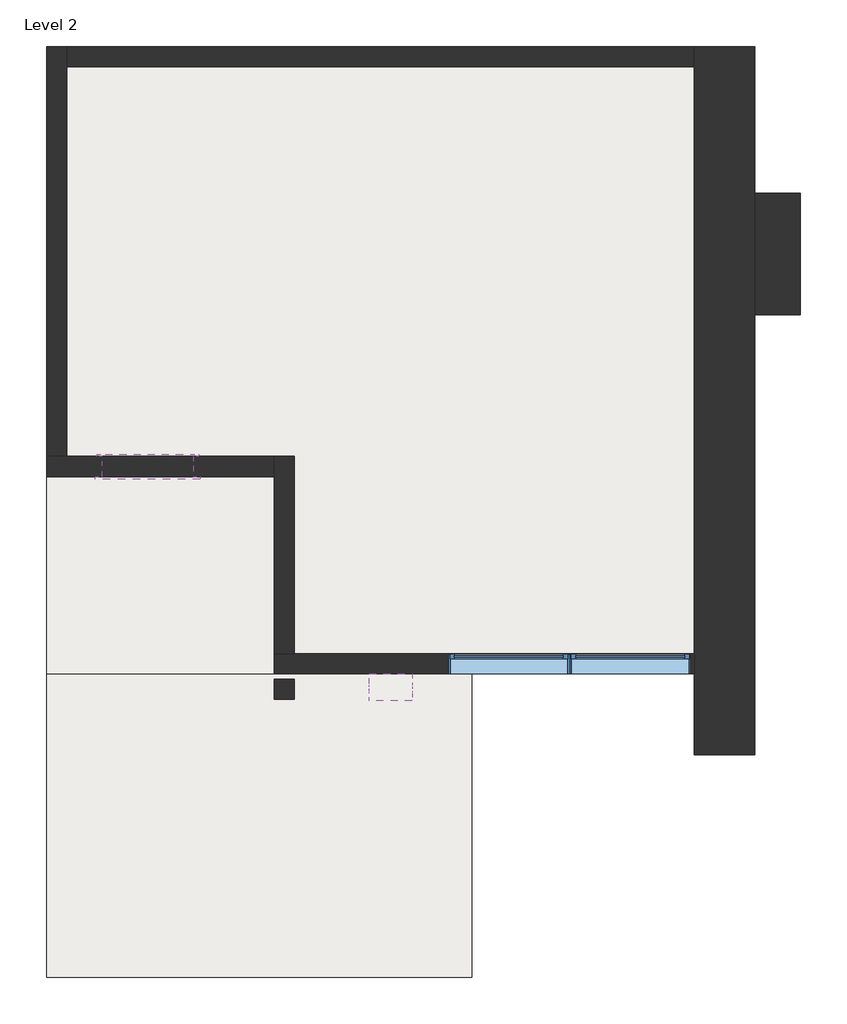
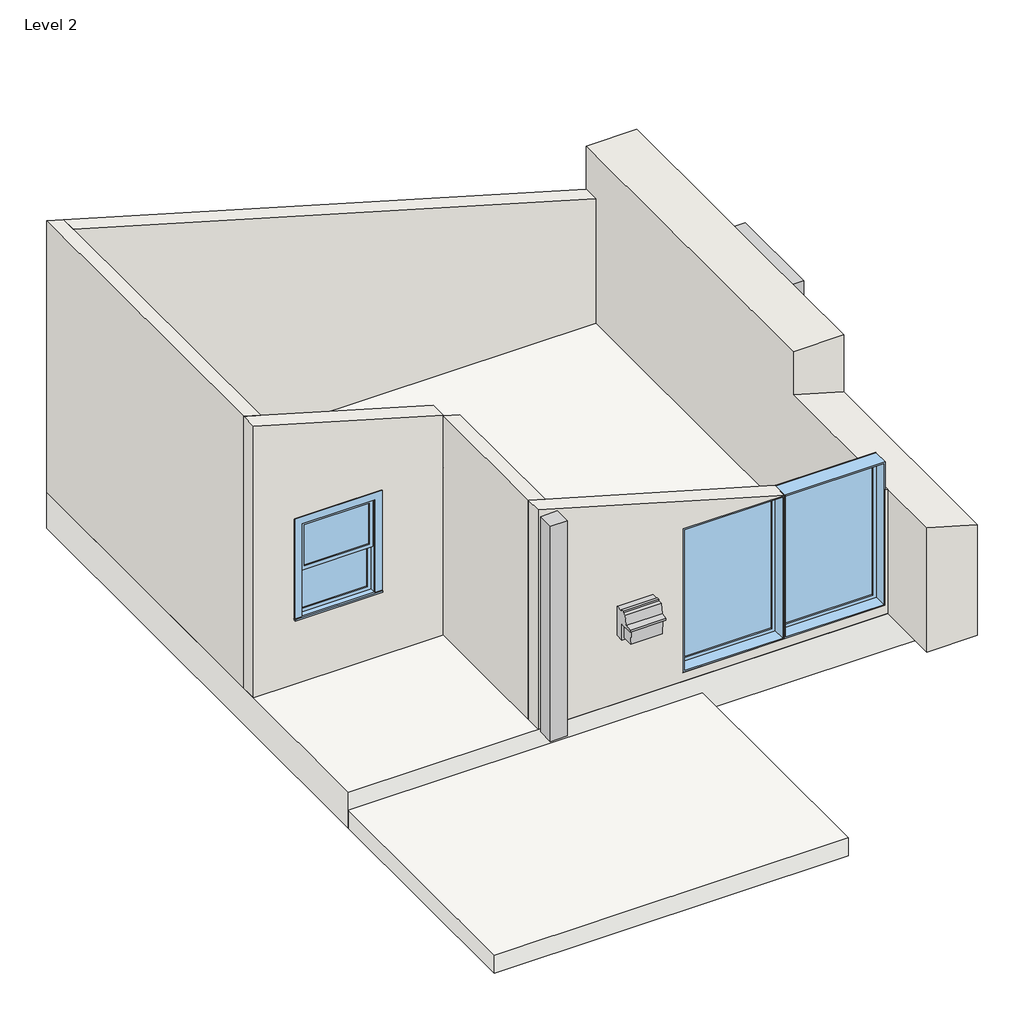
# One storey: 6 walls, 3 windows, 2 columns, 2 roofs, 1 light fixture.
"""IFC4 building model written with IfcOpenShell, lengths in millimetres."""

from ifc_helpers import new_model, si_unit, frame, origin, place, context, project, spatial, polyline, outline, extrude, faceted_brep, transform, mapped, element, save
from components import wall_pack_light_exterior_120v_50d39a1a, window_31198920, window_b4876e44

model = new_model("IFC4")

# Units and contexts
model_context = context("Model", 3, world=origin())
ifc_project = project(units=[si_unit("LENGTHUNIT", "METRE", prefix="MILLI")], contexts=[model_context])

# Site, building, storey
site = spatial("IfcSite", under=ifc_project)
building = spatial("IfcBuilding", under=site)
storey = spatial("IfcBuildingStorey", under=building, Name="Level 2", Elevation=3048.0)

# Columns
placement = place(None, origin())
element("IfcColumn", 1, ObjectType="Rectangular Column : 18\" x 18\"", at=placement, inside=storey, context=model_context, shape_type="SweptSolid", body=[
    extrude(outline(polyline([(-18066.8304544, -4040.8287936), (-18066.8304544, -4244.0287936), (-18270.0304544, -4244.0287936), (-18270.0304544, -4040.8287936), (-18066.8304544, -4040.8287936)])), frame((0.0, 0.0, 3505.2), z_axis=(0.0, 0.0, 1.0), x_axis=(1.0, 0.0, 0.0)), (0.0, 0.0, 1.0), 2743.2),
])
element("IfcColumn", 2, ObjectType="Rectangular Column : 24\" x 24\"", at=placement, inside=storey, context=model_context, shape_type="SweptSolid", body=[
    extrude(outline(polyline([(3048.0, -13901.2613196), (3048.0, -12986.8613196), (5181.6, -12986.8613196), (5181.6, -13444.0613196), (3505.2, -13444.0613196), (3505.2, -13901.2613196), (3048.0, -13901.2613196)])), frame((0.0, -381.4582127, 0.0), z_axis=(0.0, 1.0, 0.0), x_axis=(0.0, 0.0, 1.0)), (0.0, 0.0, 1.0), 1219.2),
])

# Light fixture
wall_pack_light_exterior_120v_shape = wall_pack_light_exterior_120v_50d39a1a(model_context)
element("IfcLightFixture", 3, ObjectType="Wall Pack Light - Exterior : 120V", at=placement, inside=storey, context=model_context, shape_type="MappedRepresentation", body=[
    mapped(wall_pack_light_exterior_120v_shape, transform((-16979.8972631, -3886.6582127, 1996.0613502), x_axis=(-1.0, 0.0, 0.0), y_axis=(0.0, -1.0, 0.0), z_axis=(0.0, 0.0, 1.0))),
])

# Roofs
element("IfcRoof", 4, ObjectType="Generic - 18\" 2", at=placement, inside=storey, context=model_context, shape_type="SweptSolid", body=[
    extrude(outline(polyline([(-20556.0613196, 2310.9417873), (-13444.0613196, 2310.9417873), (-13444.0613196, -3988.2582127), (-20556.0613196, -3988.2582127), (-20556.0613196, 2310.9417873)])), frame((0.0, 0.0, 3048.0), z_axis=(0.0, 0.0, 1.0), x_axis=(1.0, 0.0, 0.0)), (0.0, 0.0, 1.0), 457.2),
])
element("IfcRoof", 5, ObjectType="Generic - 9\"", at=placement, inside=storey, context=model_context, shape_type="SweptSolid", body=[
    extrude(outline(polyline([(-20556.0613196, -3988.2582127), (-16288.8613196, -3988.2582127), (-16288.8613196, -7036.2582127), (-20556.0613196, -7036.2582127), (-20556.0613196, -3988.2582127)])), frame((0.0, 0.0, 3048.0), z_axis=(0.0, 0.0, 1.0), x_axis=(1.0, 0.0, 0.0)), (0.0, 0.0, 1.0), 228.6),
])

# Walls
element("IfcWall", 6, ObjectType="Generic - 8\"", at=placement, inside=storey, context=model_context, shape_type="Brep", body=[
    faceted_brep([(-14053.6613196, -3785.0582127, 3505.2), (-18066.8613196, -3785.0582127, 3505.2), (-18270.0613196, -3785.0582127, 3505.2), (-18270.0613196, -3785.0582127, 6301.6044651), (-18066.8613196, -3785.0582127, 6243.2365005), (-15293.901566, -3785.0582127, 5446.7206706), (-16523.9413429, -3785.0582127, 5446.7206706), (-16523.9413429, -3785.0582127, 3617.9206706), (-14085.5413429, -3785.0582127, 3617.9206706), (-14085.5413429, -3785.0582127, 5099.6265433), (-14053.6613196, -3785.0582127, 5090.4692004), (-18270.0613196, -3988.2582127, 3505.2), (-14053.6613196, -3988.2582127, 3505.2), (-14053.6613196, -3988.2582127, 5090.4692004), (-14085.5413429, -3988.2582127, 5099.6265433), (-14085.5413429, -3988.2582127, 3617.9206706), (-16523.9413429, -3988.2582127, 3617.9206706), (-16523.9413429, -3988.2582127, 5446.7206706), (-15293.901566, -3988.2582127, 5446.7206706), (-18270.0613196, -3988.2582127, 6301.6044651)], [[[0, 1, 2, 3, 4, 5, 6, 7, 8, 9, 10]], [[11, 12, 13, 14, 15, 16, 17, 18, 19]], [[2, 1, 0, 12, 11]], [[3, 2, 11, 19]], [[0, 10, 13, 12]], [[8, 15, 14, 9]], [[16, 7, 6, 17]], [[7, 16, 15, 8]], [[17, 6, 5, 18]], [[3, 19, 18, 5, 4]], [[13, 10, 9, 14]]]),
])
element("IfcWall", 7, ObjectType="Generic - 8\"", at=placement, inside=storey, context=model_context, shape_type="Brep", body=[
    faceted_brep([(-18066.8613196, -3785.0582127, 3505.2), (-18066.8613196, -1803.8582127, 3505.2), (-18066.8613196, -1803.8582127, 5638.8), (-18066.8613196, -2007.0582127, 5638.8), (-18066.8613196, -2007.0582127, 6243.2365005), (-18066.8613196, -3785.0582127, 6243.2365005), (-18270.0613196, -3785.0582127, 3505.2), (-18270.0613196, -3785.0582127, 6301.6044651), (-18270.0613196, -2007.0582127, 6301.6044651), (-18270.0613196, -2007.0582127, 5638.8), (-18270.0613196, -1803.8582127, 5638.8), (-18270.0613196, -1803.8582127, 3505.2), (-18270.0613196, -2007.0582127, 3505.2)], [[[0, 1, 2, 3, 4, 5]], [[6, 7, 8, 9, 10, 11, 12]], [[1, 0, 6, 12, 11]], [[0, 5, 7, 6]], [[2, 1, 11, 10]], [[3, 2, 10, 9]], [[3, 9, 8, 4]], [[5, 4, 8, 7]]]),
])
element("IfcWall", 8, ObjectType="Generic - 8\"", at=placement, inside=storey, context=model_context, shape_type="Brep", body=[
    faceted_brep([(-18270.0613196, -1803.8582127, 3505.2), (-20352.8613196, -1803.8582127, 3505.2), (-20556.0613196, -1803.8582127, 3505.2), (-20556.0613196, -1803.8582127, 6966.6625001), (-20352.8613196, -1803.8582127, 6908.0886191), (-18270.0613196, -1803.8582127, 6307.7063391), (-18270.0613196, -1803.8582127, 5638.8), (-19997.2613196, -1803.8582127, 5544.8047365), (-19997.2613196, -1803.8582127, 4325.6047365), (-19082.8613196, -1803.8582127, 4325.6047365), (-19082.8613196, -1803.8582127, 5544.8047365), (-18270.0613196, -2007.0582127, 3505.2), (-18270.0613196, -2007.0582127, 6307.7063391), (-20556.0613196, -2007.0582127, 6966.6625001), (-20556.0613196, -2007.0582127, 3505.2), (-19997.2613196, -2007.0582127, 5544.8047365), (-19082.8613196, -2007.0582127, 5544.8047365), (-19082.8613196, -2007.0582127, 4325.6047365), (-19997.2613196, -2007.0582127, 4325.6047365)], [[[0, 1, 2, 3, 4, 5, 6], [7, 8, 9, 10]], [[11, 12, 13, 14], [15, 16, 17, 18]], [[2, 1, 0, 11, 14]], [[0, 6, 5, 12, 11]], [[3, 2, 14, 13]], [[5, 4, 3, 13, 12]], [[8, 7, 15, 18]], [[9, 8, 18, 17]], [[10, 9, 17, 16]], [[7, 10, 16, 15]]]),
])
element("IfcWall", 9, ObjectType="Generic - 8\"", at=placement, inside=storey, context=model_context, shape_type="Brep", body=[
    faceted_brep([(-20352.8613196, -1803.8582127, 3505.2), (-20352.8613196, 2107.7417873, 3505.2), (-20352.8613196, 2310.9417873, 3505.2), (-20352.8613196, 2310.9417873, 6908.0886191), (-20352.8613196, 2107.7417873, 6908.0886191), (-20352.8613196, -1803.8582127, 6908.0886191), (-20556.0613196, -1803.8582127, 3505.2), (-20556.0613196, -1803.8582127, 6966.6625001), (-20556.0613196, 2310.9417873, 6966.6625001), (-20556.0613196, 2310.9417873, 3505.2)], [[[0, 1, 2, 3, 4, 5]], [[6, 7, 8, 9]], [[2, 1, 0, 6, 9]], [[0, 5, 7, 6]], [[3, 2, 9, 8]], [[5, 4, 3, 8, 7]]]),
])
element("IfcWall", 10, ObjectType="Generic - 8\"", at=placement, inside=storey, context=model_context, shape_type="SweptSolid", body=[
    extrude(outline(polyline([(3505.2, -20352.8613196), (3505.2, -14053.6613196), (5092.2983086, -14053.6613196), (6908.0886191, -20352.8613196), (3505.2, -20352.8613196)])), frame((0.0, 2107.7417873, 0.0), z_axis=(0.0, 1.0, 0.0), x_axis=(0.0, 0.0, 1.0)), (0.0, 0.0, 1.0), 203.2),
])
element("IfcWall", 11, ObjectType="Generic - 8\" 2", at=placement, inside=storey, context=model_context, shape_type="Brep", body=[
    faceted_brep([(-14053.6613196, 2310.9417873, 3505.2), (-14053.6613196, 2107.7417873, 3505.2), (-14053.6613196, -3785.0582127, 3505.2), (-14053.6613196, -3988.2582127, 3505.2), (-14053.6613196, -4801.0582127, 3505.2), (-14053.6613196, -4801.0582127, 5090.4692004), (-14053.6613196, -3988.2582127, 5090.4692004), (-14053.6613196, -3785.0582127, 5090.4692004), (-14053.6613196, -2007.0582127, 5090.4692004), (-14053.6613196, -2007.0582127, 5638.8), (-14053.6613196, -279.8582127, 5638.8), (-14053.6613196, 634.5417873, 5638.8), (-14053.6613196, 2310.9417873, 5638.8), (-14053.6613196, 2310.9417873, 5092.2983086), (-13444.0613196, 2310.9417873, 3505.2), (-13444.0613196, 2310.9417873, 5638.8), (-13444.0613196, 634.5417873, 5638.8), (-13444.0613196, -279.8582127, 5638.8), (-13444.0613196, -2007.0582127, 5638.8), (-13444.0613196, -2007.0582127, 4915.3653067), (-13444.0613196, -4801.0582127, 4915.3653067), (-13444.0613196, -4801.0582127, 3505.2), (-13444.0613196, -381.4582127, 3505.2), (-13444.0613196, 837.7417873, 3505.2)], [[[0, 1, 2, 3, 4, 5, 6, 7, 8, 9, 10, 11, 12, 13]], [[14, 15, 16, 17, 18, 19, 20, 21, 22, 23]], [[4, 3, 2, 1, 0, 14, 23, 22, 21]], [[5, 4, 21, 20]], [[0, 13, 12, 15, 14]], [[12, 11, 10, 9, 18, 17, 16, 15]], [[18, 9, 8, 19]], [[8, 7, 6, 5, 20, 19]]]),
])

# Windows
window_shape = window_31198920(model_context)
element("IfcWindow", 12, ObjectType="Double Hung with Trim : 36\" x 48\"", at=placement, inside=storey, context=model_context, shape_type="MappedRepresentation", body=[
    mapped(window_shape, transform((-19540.0613196, -1905.4582127, 3411.2047365), x_axis=(-1.0, 0.0, 0.0), y_axis=(0.0, -1.0, 0.0), z_axis=(0.0, 0.0, 1.0))),
])
window_2_shape = window_b4876e44(model_context)
element("IfcWindow", 13, ObjectType="Fixed : 48\" x 72\"", at=placement, inside=storey, context=model_context, shape_type="MappedRepresentation", body=[
    mapped(window_2_shape, transform((-14733.2413429, -3886.6582127, 3313.1206706), x_axis=(-1.0, 0.0, 0.0), y_axis=(0.0, -1.0, 0.0), z_axis=(0.0, 0.0, 1.0))),
])
element("IfcWindow", 14, ObjectType="Fixed : 48\" x 72\"", at=placement, inside=storey, context=model_context, shape_type="MappedRepresentation", body=[
    mapped(window_2_shape, transform((-15952.4413429, -3886.6582127, 3313.1206706), x_axis=(-1.0, 0.0, 0.0), y_axis=(0.0, -1.0, 0.0), z_axis=(0.0, 0.0, 1.0))),
])

save(model, "model.ifc")

# Revit data of these elements
# Type "Rectangular Column : 18\" x 18\""
#   Assembly Code = "B1010200"
#   Depth = 0' - 8"
#   Offset Base = 0' - 0"
#   Offset Top = 0' - 0"
#   Width = 0' - 8"
#   Material = Stainless Steel
# Type "Rectangular Column : 24\" x 24\""
#   Assembly Code = "B1010200"
#   Depth = 3' - 0"
#   Offset Base = 0' - 0"
#   Offset Top = 0' - 0"
#   Width = 4' - 0"
#   Material = none
# Type "Wall Pack Light - Exterior : 120V"
#   Assembly Code = "D5020230"
#   Wattage = 70 W
#   built-in parameter 1150110 = 1 (stored number, unit not read)
#   built-in parameter 1114217 = 1 (stored number, unit not read)
#   built-in parameter 1150109 = 1 (stored number, unit not read)
#   built-in parameter 1150113 = 1 (stored number, unit not read)
#   built-in parameter 1150115 = 1 (stored number, unit not read)
#   built-in parameter 1150105 = 437.668 (stored number, unit not read)
#   Light Source Symbol Size = 2' - 0"
#   built-in parameter 1150112 = 1 (stored number, unit not read)
#   built-in parameter 1150114 = 1 (stored number, unit not read)
#   built-in parameter 1150107 = 4000 (stored number, unit not read)
#   built-in parameter 1150106 = 4.37668 (stored number, unit not read)
#   built-in parameter 1150104 = 7.29939 (stored number, unit not read)
#   Ballast Voltage = 120 V
#   built-in parameter 1114218 = 1 (stored number, unit not read)
#   built-in parameter 1150133 = 10 (stored number, unit not read)
#   Lumens = 5499.9 lm
#   Mounting Height = 9' - 0"
#   Apparent Load = 70 VA
#   built-in parameter 1150134 = 12
#   built-in parameter 1150137 = 1
#   Color Filter = 16777215
#   Ballast Number of Poles = 1
#   Wall Mount Material = Metal - Paint Finish - Dark Grey, Matte
#   Shade Material = Glass
#   Load Classification = Lighting - Exterior
#   Dimming Lamp Color Temperature Shift = (empty or 0)
#   Default Elevation = 0
# Type "Generic - 18\" 2"
#   Assembly Code = "B1020"
#   Layers, outside or top first: 1' - 6" "Stainless Steel" (function 1)
# Type "Generic - 9\""
#   Assembly Code = "B1020"
#   Layers, outside or top first: 0' - 9" "Stainless Steel" (function 1)
# Type "Generic - 8\""
#   Assembly Code = "B2010"
#   Layers, outside or top first: 0' - 8" "Brick, Soldier Course" (function 1)
# Type "Generic - 8\" 2"
#   Assembly Code = "B2010"
#   Layers, outside or top first: 2' - 0" "Brick, Soldier Course" (function 1)
# Type "Double Hung with Trim : 36\" x 48\""
#   Type Mark = "15"
#   Construction Type Id = "GSP4R"
#   Assembly Code = "B2020100"
#   Analytic Construction = "1/8 in Pilkington single glazing"
#   Visual Light Transmittance = 0.9
#   Solar Heat Gain Coefficient = 0.78
#   Heat Transfer Coefficient (U) = 0.6496 BTU/(h·ft²·°F)
#   Height = 4' - 0"
#   Default Sill Height = 3' - 0"
#   Trim Projection - Ext. = 0' - 0 1/2"
#   Trim Projection - Int. = 0' - 0 3/4"
#   Trim Width - Exterior = 0' - 3 1/2"
#   Trim Width - Interior = 0' - 3 1/2"
#   Width = 3' - 0"
#   Window Inset = 0' - 0 3/4"
#   Define Thermal Properties by = 1
#   Glass Pane Material = Glass
#   Sash Material = Structure, Steel Bar Joist Layer
#   Trim Exterior Material = Vapor Retarder
#   Trim Interior Material = Vapor Retarder
#   Wall Closure = (empty or 0)
# Type "Fixed : 48\" x 72\""
#   Type Mark = "13"
#   Construction Type Id = "GSP4R"
#   Assembly Code = "B2020100"
#   Analytic Construction = "1/8 in Pilkington single glazing"
#   Visual Light Transmittance = 0.9
#   Solar Heat Gain Coefficient = 0.78
#   Heat Transfer Coefficient (U) = 0.6496 BTU/(h·ft²·°F)
#   Height = 6' - 0"
#   Default Sill Height = 1' - 0"
#   Width = 4' - 0"
#   Window Inset = 0' - 6"
#   Define Thermal Properties by = 1
#   Glass Pane Material = Glass
#   Sash Material = Structure, Steel Bar Joist Layer
#   Wall Closure = (empty or 0)
# Element 1 (IfcColumn, "Rectangular Column : 18\" x 18\"")
#   Phase Created = New Construction
#   Materials on its faces: "Stainless Steel"
# Element 2 (IfcColumn, "Rectangular Column : 24\" x 24\"")
#   Phase Created = New Construction
#   Materials on its faces: "Oak Flooring", "Brick, Soldier Course"
# Element 3 (IfcLightFixture, "Wall Pack Light - Exterior : 120V")
#   Mark = "4"
#   Phase Created = New Construction
#   Materials on its faces: "Metal - Paint Finish - Dark Grey, Matte", "Glass"
# Element 4 (IfcRoof, "Generic - 18\" 2")
#   built-in parameter 1001705 = 11.5 (stored number, unit not read)
#   built-in parameter 1001710 = 33615
#   Phase Created = New Construction
#   Materials on its faces: "Stainless Steel", "Rigid insulation"
# Element 5 (IfcRoof, "Generic - 9\"")
#   built-in parameter 1001705 = 10.75 (stored number, unit not read)
#   built-in parameter 1001710 = 33615
#   Phase Created = New Construction
#   Materials on its faces: "Stainless Steel", "Cherry", "Rigid insulation"
# Elements 6, 8, 9 (IfcWall, "Generic - 8\"")
#   built-in parameter 1001111 = 1' - 6"
#   Top Offset = 0' - 0"
#   Base Offset = 1' - 6"
#   Unconnected Height = 7' - 0"
#   wall height = 7' - 0"
#   Phase Created = New Construction
#   Base Constraint = Level 2
#   Materials on its faces: "Brick, Soldier Course", "Oak Flooring", "Rigid insulation"
# Elements 7, 10 (IfcWall, "Generic - 8\"")
#   built-in parameter 1001111 = 1' - 6"
#   Top Offset = 0' - 0"
#   Base Offset = 1' - 6"
#   Unconnected Height = 7' - 0"
#   wall height = 7' - 0"
#   Phase Created = New Construction
#   Base Constraint = Level 2
#   Materials on its faces: "Brick, Soldier Course", "Rigid insulation", "Oak Flooring"
# Element 11 (IfcWall, "Generic - 8\" 2")
#   built-in parameter 1001111 = 1' - 6"
#   Top Offset = 0' - 0"
#   Base Offset = 1' - 6"
#   Unconnected Height = 7' - 0"
#   wall height = 7' - 0"
#   Phase Created = New Construction
#   Base Constraint = Level 2
#   Materials on its faces: "Brick, Soldier Course", "Oak Flooring", "Rigid insulation"
# Element 12 (IfcWindow, "Double Hung with Trim : 36\" x 48\"")
#   Mark = "8"
#   Phase Created = New Construction
#   Materials on its faces: "Structure, Steel Bar Joist Layer", "Vapor Retarder", "Glass"
# Element 13 (IfcWindow, "Fixed : 48\" x 72\"")
#   Mark = "6"
#   Phase Created = New Construction
#   Materials on its faces: "Structure, Steel Bar Joist Layer", "Glass"
# Element 14 (IfcWindow, "Fixed : 48\" x 72\"")
#   Mark = "7"
#   Phase Created = New Construction
#   Materials on its faces: "Structure, Steel Bar Joist Layer", "Glass"
# Materials
#   "Stainless Steel": class "Metal", colour RGB 0 0 0, transparency 0, Description = "Stainless Steel 18/8", Cost = 0
#   "Metal - Paint Finish - Dark Grey, Matte": class "Paint", colour RGB 98 98 98, transparency 0
#   "Glass": class "Glass", colour RGB 0 128 192, transparency 0.75, Description = "Soda Lime Glass", Cost = 0
#   "Brick, Soldier Course": class "Masonry", colour RGB 170 98 104, transparency 0, Description = "Common brick soldier coursed", Cost = 0
#   "Structure, Steel Bar Joist Layer": class "Metal", colour RGB 127 127 127, transparency 0, Description = "Bar joists, thermal airspace", Cost = 0
#   "Vapor Retarder": class "Generic", colour RGB 127 127 127, transparency 0, Description = "Polyethylene film membrane", Cost = 0
#   "Oak Flooring": class "Wood", colour RGB 216 169 114, transparency 0, Description = "Quercus Rubra", Cost = 0
#   "Rigid insulation": class "Generic", colour RGB 127 127 127, transparency 0, Description = "Rigid foam insulation board", Cost = 0
#   "Cherry": class "Wood", colour RGB 226 177 128, transparency 0, Description = "Prunus Serotina", Cost = 0
